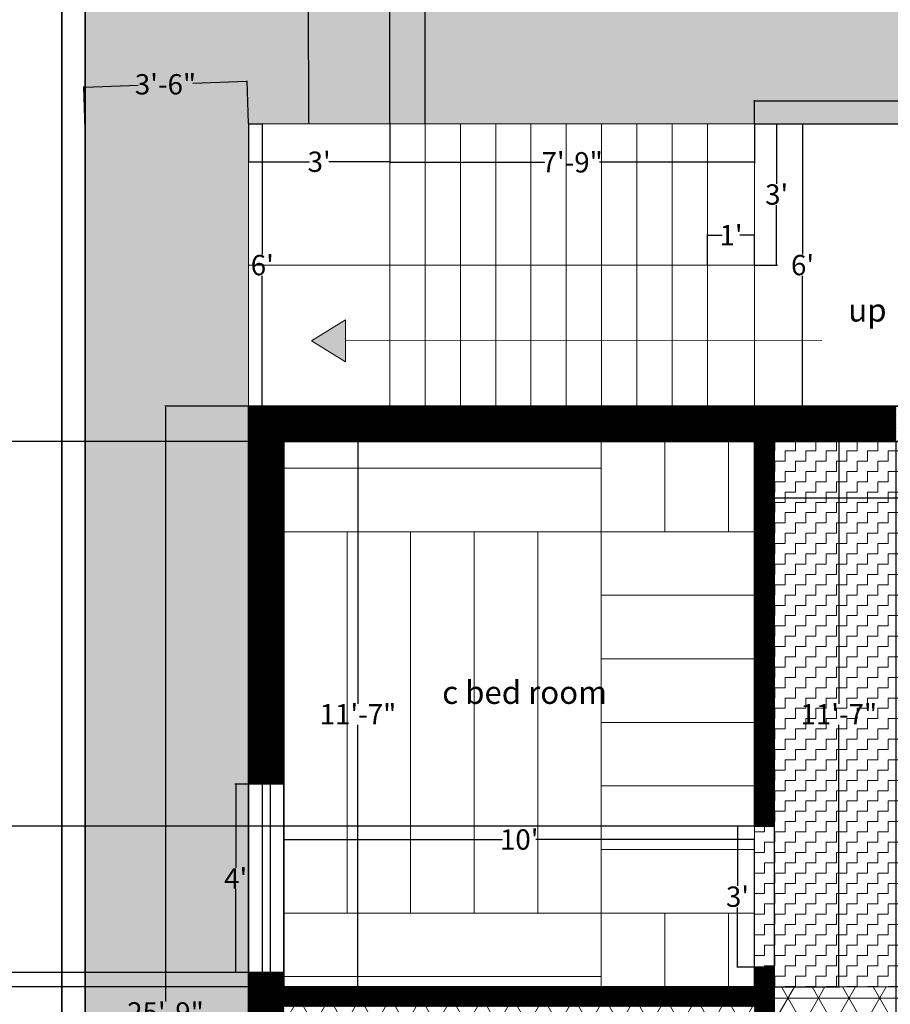
# Model space of a CAD drawing. Units: inches. Extents: x -157 to 1464, y -361 to 1077.
# Tile 5 of 9: x 241 to 463, y 268 to 519. Entities that reach past the tile are written whole.
import ezdxf

# ---------------------------------------------------------------- set-up
doc = ezdxf.new("R2010")
doc.units = ezdxf.units.IN
doc.header["$MEASUREMENT"] = 0
for name, color, linetype, lineweight in [('A-ANNO-DIMS', 2, 'Continuous', 18), ('A-ANNO-SYMB', 7, 'Continuous', 18), ('A-ANNO-SYMB-PATT', 7, 'Continuous', 13), ('A-ANNO-TEXT', 7, 'Continuous', 18), ('A-AREA-IDEN', 7, 'Continuous', 18), ('A-FLOR', 7, 'Continuous', 25), ('A-FLOR-BNDY', 9, 'Continuous', 13), ('A-FLOR-PATT', 8, 'Continuous', 13), ('A-FLOR-STRS', 7, 'Continuous', 18), ('A-WALL', 7, 'Continuous', 35), ('A-WALL-PATT', 252, 'Continuous', 13), ('C-ANNO-DIMS', 2, 'Continuous', 18), ('C-PROP', 7, 'Continuous', 35), ('doors and windows', 33, 'Continuous', 25), ('L-GRND-PATT', 8, 'Continuous', 13)]:
    doc.layers.add(name, color=color, linetype=linetype, lineweight=lineweight)
doc.styles.get("Standard").update_dxf_attribs({"font": 'arial.ttf'})
doc.dimstyles.new('Annotative', dxfattribs={"dimscale": 0, "dimtxt": 5.18, "dimasz": 0.18, "dimexe": 0.18, "dimexo": 0.0625, "dimgap": 0.09, "dimtad": 0, "dimtih": 1, "dimtoh": 1, "dimdec": 0, "dimzin": 0, "dimdsep": 46, "dimlunit": 3, "dimtxsty": 'Standard', "dimcen": 0.09, "dimadec": 0, "dimazin": 0, "dimtfac": 1, "dimtdec": 0, "dimtofl": 0, "dimtmove": 0, "dimatfit": 3, "dimfxl": 1, "dimtolj": 1, "dimtzin": 0, "dimarcsym": 0})

# ---------------------------------------------------------------- blocks, each defined once
blk = doc.blocks.new('*D1')
at = {"layer": 'A-ANNO-DIMS', "color": 0, "lineweight": -2, "transparency": 16777216}
for p, q in [((298.9, 420.86), (277.62, 420.86)), ((277.8, 420.68), (277.8, 269.1)), ((277.8, 112.04), (277.8, 263.63)), ((298.9, 111.86), (277.62, 111.86))]:
    blk.add_line(p, q, dxfattribs=at)
at = {"layer": 'A-ANNO-DIMS', "color": 0, "transparency": 16777216}
for points in [[(277.77, 420.68), (277.83, 420.68), (277.8, 420.86)], [(277.77, 112.04), (277.83, 112.04), (277.8, 111.86)]]:
    blk.add_solid(points, dxfattribs=at)
at = {"layer": 'Defpoints', "color": 0, "transparency": 16777216}
for p in [(298.97, 420.86), (277.8, 111.86), (298.97, 111.86)]:
    blk.add_point(p, dxfattribs=at)
at = {"layer": 'A-ANNO-DIMS', "color": 0, "transparency": 16777216, "insert": (277.8, 266.36), "char_height": 5.18, "attachment_point": 5}
blk.add_mtext('\\A1;25\'-9"', dxfattribs=at)
blk = doc.blocks.new('*D7')
at = {"layer": 'A-ANNO-DIMS', "color": 0, "lineweight": -2, "transparency": 16777216}
for p, q in [((307.97, 272.92), (307.97, 310.62)), ((308.15, 310.44), (363.72, 310.44)), ((427.79, 310.44), (372.21, 310.44)), ((427.97, 272.92), (427.97, 310.62))]:
    blk.add_line(p, q, dxfattribs=at)
at = {"layer": 'A-ANNO-DIMS', "color": 0, "transparency": 16777216}
for points in [[(308.15, 310.47), (308.15, 310.41), (307.97, 310.44)], [(427.79, 310.47), (427.79, 310.41), (427.97, 310.44)]]:
    blk.add_solid(points, dxfattribs=at)
at = {"layer": 'Defpoints', "color": 0, "transparency": 16777216}
for p in [(427.97, 310.44), (307.97, 272.86), (427.97, 272.86)]:
    blk.add_point(p, dxfattribs=at)
at = {"layer": 'A-ANNO-DIMS', "color": 0, "transparency": 16777216, "insert": (367.97, 310.44), "char_height": 5.18, "attachment_point": 5}
blk.add_mtext("\\A1;10'", dxfattribs=at)
blk = doc.blocks.new('*D8')
at = {"layer": 'A-ANNO-DIMS', "color": 0, "lineweight": -2, "transparency": 16777216}
for p, q in [((308.03, 411.86), (327.05, 411.86)), ((326.87, 411.68), (326.87, 345.05)), ((326.87, 273.04), (326.87, 339.67)), ((308.03, 272.86), (327.05, 272.86))]:
    blk.add_line(p, q, dxfattribs=at)
at = {"layer": 'A-ANNO-DIMS', "color": 0, "transparency": 16777216}
for points in [[(326.84, 411.68), (326.9, 411.68), (326.87, 411.86)], [(326.84, 273.04), (326.9, 273.04), (326.87, 272.86)]]:
    blk.add_solid(points, dxfattribs=at)
at = {"layer": 'Defpoints', "color": 0, "transparency": 16777216}
for p in [(307.97, 411.86), (326.87, 411.86), (307.97, 272.86)]:
    blk.add_point(p, dxfattribs=at)
at = {"layer": 'A-ANNO-DIMS', "color": 0, "transparency": 16777216, "insert": (326.87, 342.36), "char_height": 5.18, "attachment_point": 5}
blk.add_mtext('\\A1;11\'-7"', dxfattribs=at)
blk = doc.blocks.new('*D13')
at = {"layer": 'C-ANNO-DIMS', "color": 0, "lineweight": -2, "transparency": 16777216}
for p, q in [((257.27, 643.42), (188.08, 643.42)), ((188.26, 643.24), (188.26, 359.63)), ((188.26, 70.55), (188.26, 354.16)), ((257.27, 70.37), (188.08, 70.37))]:
    blk.add_line(p, q, dxfattribs=at)
at = {"layer": 'C-ANNO-DIMS', "color": 0, "transparency": 16777216}
for points in [[(188.23, 643.24), (188.29, 643.24), (188.26, 643.42)], [(188.23, 70.55), (188.29, 70.55), (188.26, 70.37)]]:
    blk.add_solid(points, dxfattribs=at)
at = {"layer": 'Defpoints', "color": 0, "transparency": 16777216}
for p in [(257.33, 643.42), (188.26, 70.37), (257.33, 70.37)]:
    blk.add_point(p, dxfattribs=at)
at = {"layer": 'C-ANNO-DIMS', "color": 0, "transparency": 16777216, "insert": (188.26, 356.89), "char_height": 5.18, "attachment_point": 5}
blk.add_mtext('\\A1;47\'-9"', dxfattribs=at)
blk = doc.blocks.new('*D18')
at = {"layer": 'A-ANNO-DIMS', "color": 0, "lineweight": -2, "transparency": 16777216}
for p, q in [((298.97, 492.8), (298.97, 483.03)), ((334.97, 492.8), (334.97, 483.03)), ((299.15, 483.21), (314.5, 483.21)), ((334.79, 483.21), (319.44, 483.21))]:
    blk.add_line(p, q, dxfattribs=at)
at = {"layer": 'A-ANNO-DIMS', "color": 0, "transparency": 16777216}
for points in [[(299.15, 483.24), (299.15, 483.18), (298.97, 483.21)], [(334.79, 483.24), (334.79, 483.18), (334.97, 483.21)]]:
    blk.add_solid(points, dxfattribs=at)
at = {"layer": 'Defpoints', "color": 0, "transparency": 16777216}
for p in [(298.97, 492.86), (334.97, 492.86), (334.97, 483.21)]:
    blk.add_point(p, dxfattribs=at)
at = {"layer": 'A-ANNO-DIMS', "color": 0, "transparency": 16777216, "insert": (316.97, 483.21), "char_height": 5.18, "attachment_point": 5}
blk.add_mtext("\\A1;3'", dxfattribs=at)
blk = doc.blocks.new('*D19')
at = {"layer": 'A-ANNO-DIMS', "color": 0, "lineweight": -2, "transparency": 16777216}
for p, q in [((334.97, 492.8), (334.97, 482.88)), ((427.97, 492.8), (427.97, 482.88)), ((335.15, 483.06), (374.51, 483.06)), ((427.79, 483.06), (388.42, 483.06))]:
    blk.add_line(p, q, dxfattribs=at)
at = {"layer": 'A-ANNO-DIMS', "color": 0, "transparency": 16777216}
for points in [[(335.15, 483.09), (335.15, 483.03), (334.97, 483.06)], [(427.79, 483.09), (427.79, 483.03), (427.97, 483.06)]]:
    blk.add_solid(points, dxfattribs=at)
at = {"layer": 'Defpoints', "color": 0, "transparency": 16777216}
for p in [(334.97, 492.86), (427.97, 492.86), (427.97, 483.06)]:
    blk.add_point(p, dxfattribs=at)
at = {"layer": 'A-ANNO-DIMS', "color": 0, "transparency": 16777216, "insert": (381.47, 483.06), "char_height": 5.18, "attachment_point": 5}
blk.add_mtext('\\A1;7\'-9"', dxfattribs=at)
blk = doc.blocks.new('*D20')
at = {"layer": 'A-ANNO-DIMS', "color": 0, "lineweight": -2, "transparency": 16777216}
for p, q in [((299.03, 492.86), (302.65, 492.86)), ((302.47, 492.68), (302.47, 459.6)), ((302.47, 421.04), (302.47, 454.13)), ((299.03, 420.86), (302.65, 420.86))]:
    blk.add_line(p, q, dxfattribs=at)
at = {"layer": 'A-ANNO-DIMS', "color": 0, "transparency": 16777216}
for points in [[(302.44, 492.68), (302.5, 492.68), (302.47, 492.86)], [(302.44, 421.04), (302.5, 421.04), (302.47, 420.86)]]:
    blk.add_solid(points, dxfattribs=at)
at = {"layer": 'Defpoints', "color": 0, "transparency": 16777216}
for p in [(298.97, 492.86), (302.47, 492.86), (298.97, 420.86)]:
    blk.add_point(p, dxfattribs=at)
at = {"layer": 'A-ANNO-DIMS', "color": 0, "transparency": 16777216, "insert": (302.47, 456.86), "char_height": 5.18, "attachment_point": 5}
blk.add_mtext("\\A1;6'", dxfattribs=at)
blk = doc.blocks.new('*D21')
at = {"layer": 'A-ANNO-DIMS', "color": 0, "lineweight": -2, "transparency": 16777216}
for p, q in [((428.03, 492.86), (440.38, 492.86)), ((440.2, 492.68), (440.2, 459.6)), ((440.2, 421.04), (440.2, 454.13)), ((428.03, 420.86), (440.38, 420.86))]:
    blk.add_line(p, q, dxfattribs=at)
at = {"layer": 'A-ANNO-DIMS', "color": 0, "transparency": 16777216}
for points in [[(440.17, 492.68), (440.23, 492.68), (440.2, 492.86)], [(440.17, 421.04), (440.23, 421.04), (440.2, 420.86)]]:
    blk.add_solid(points, dxfattribs=at)
at = {"layer": 'Defpoints', "color": 0, "transparency": 16777216}
for p in [(427.97, 492.86), (427.97, 420.86), (440.2, 420.86)]:
    blk.add_point(p, dxfattribs=at)
at = {"layer": 'A-ANNO-DIMS', "color": 0, "transparency": 16777216, "insert": (440.2, 456.86), "char_height": 5.18, "attachment_point": 5}
blk.add_mtext("\\A1;6'", dxfattribs=at)
blk = doc.blocks.new('*D24')
at = {"layer": 'A-ANNO-DIMS', "color": 0, "lineweight": -2, "transparency": 16777216}
for p, q in [((432.97, 411.8), (432.97, 397.39)), ((587.97, 411.8), (587.97, 397.39)), ((433.15, 397.57), (499.71, 397.57)), ((587.79, 397.57), (521.22, 397.57))]:
    blk.add_line(p, q, dxfattribs=at)
at = {"layer": 'A-ANNO-DIMS', "color": 0, "transparency": 16777216}
for points in [[(433.15, 397.6), (433.15, 397.54), (432.97, 397.57)], [(587.79, 397.6), (587.79, 397.54), (587.97, 397.57)]]:
    blk.add_solid(points, dxfattribs=at)
at = {"layer": 'Defpoints', "color": 0, "transparency": 16777216}
for p in [(432.97, 411.86), (587.97, 411.86), (587.97, 397.57)]:
    blk.add_point(p, dxfattribs=at)
at = {"layer": 'A-ANNO-DIMS', "color": 0, "transparency": 16777216, "insert": (510.47, 397.57), "char_height": 5.18, "attachment_point": 5}
blk.add_mtext('\\A1;12\'-11"', dxfattribs=at)
blk = doc.blocks.new('*D25')
at = {"layer": 'A-ANNO-DIMS', "color": 0, "lineweight": -2, "transparency": 16777216}
for p, q in [((433.03, 411.86), (449.62, 411.86)), ((449.44, 411.68), (449.44, 345.05)), ((449.44, 273.04), (449.44, 339.67)), ((433.03, 272.86), (449.62, 272.86))]:
    blk.add_line(p, q, dxfattribs=at)
at = {"layer": 'A-ANNO-DIMS', "color": 0, "transparency": 16777216}
for points in [[(449.41, 411.68), (449.47, 411.68), (449.44, 411.86)], [(449.41, 273.04), (449.47, 273.04), (449.44, 272.86)]]:
    blk.add_solid(points, dxfattribs=at)
at = {"layer": 'Defpoints', "color": 0, "transparency": 16777216}
for p in [(432.97, 411.86), (432.97, 272.86), (449.44, 272.86)]:
    blk.add_point(p, dxfattribs=at)
at = {"layer": 'A-ANNO-DIMS', "color": 0, "transparency": 16777216, "insert": (449.44, 342.36), "char_height": 5.18, "attachment_point": 5}
blk.add_mtext('\\A1;11\'-7"', dxfattribs=at)
blk = doc.blocks.new('*D34')
at = {"layer": 'A-ANNO-DIMS', "color": 0, "lineweight": -2, "transparency": 16777216}
for p, q in [((302.4, 324.53), (295.51, 324.53)), ((295.69, 324.35), (295.69, 303.21)), ((295.69, 276.71), (295.69, 297.85)), ((302.4, 276.53), (295.51, 276.53))]:
    blk.add_line(p, q, dxfattribs=at)
at = {"layer": 'A-ANNO-DIMS', "color": 0, "transparency": 16777216}
for points in [[(295.66, 324.35), (295.72, 324.35), (295.69, 324.53)], [(295.66, 276.71), (295.72, 276.71), (295.69, 276.53)]]:
    blk.add_solid(points, dxfattribs=at)
at = {"layer": 'Defpoints', "color": 0, "transparency": 16777216}
for p in [(302.47, 324.53), (295.69, 276.53), (302.47, 276.53)]:
    blk.add_point(p, dxfattribs=at)
at = {"layer": 'A-ANNO-DIMS', "color": 0, "transparency": 16777216, "insert": (295.69, 300.53), "char_height": 5.18, "attachment_point": 5}
blk.add_mtext("\\A1;4'", dxfattribs=at)
blk = doc.blocks.new('*D36')
at = {"layer": 'A-ANNO-DIMS', "color": 0, "lineweight": -2, "transparency": 16777216}
for p, q in [((415.97, 456.92), (415.97, 464.68)), ((416.15, 464.5), (419.74, 464.5)), ((427.79, 464.5), (424.2, 464.5)), ((427.97, 456.92), (427.97, 464.68))]:
    blk.add_line(p, q, dxfattribs=at)
at = {"layer": 'A-ANNO-DIMS', "color": 0, "transparency": 16777216}
for points in [[(416.15, 464.53), (416.15, 464.47), (415.97, 464.5)], [(427.79, 464.53), (427.79, 464.47), (427.97, 464.5)]]:
    blk.add_solid(points, dxfattribs=at)
at = {"layer": 'Defpoints', "color": 0, "transparency": 16777216}
for p in [(427.97, 464.5), (415.97, 456.86), (427.97, 456.86)]:
    blk.add_point(p, dxfattribs=at)
at = {"layer": 'A-ANNO-DIMS', "color": 0, "transparency": 16777216, "insert": (421.97, 464.5), "char_height": 5.18, "attachment_point": 5}
blk.add_mtext("\\A1;1'", dxfattribs=at)
blk = doc.blocks.new('*D37')
at = {"layer": 'A-ANNO-DIMS', "color": 0, "lineweight": -2, "transparency": 16777216}
for p, q in [((428.03, 492.86), (433.78, 492.86)), ((433.6, 492.68), (433.6, 477.6)), ((433.6, 457.04), (433.6, 472.12)), ((428.03, 456.86), (433.78, 456.86))]:
    blk.add_line(p, q, dxfattribs=at)
at = {"layer": 'A-ANNO-DIMS', "color": 0, "transparency": 16777216}
for points in [[(433.57, 492.68), (433.63, 492.68), (433.6, 492.86)], [(433.57, 457.04), (433.63, 457.04), (433.6, 456.86)]]:
    blk.add_solid(points, dxfattribs=at)
at = {"layer": 'Defpoints', "color": 0, "transparency": 16777216}
for p in [(427.97, 492.86), (427.97, 456.86), (433.6, 456.86)]:
    blk.add_point(p, dxfattribs=at)
at = {"layer": 'A-ANNO-DIMS', "color": 0, "transparency": 16777216, "insert": (433.6, 474.86), "char_height": 5.18, "attachment_point": 5}
blk.add_mtext("\\A1;3'", dxfattribs=at)
blk = doc.blocks.new('*D50')
at = {"layer": 'A-ANNO-DIMS', "color": 0, "lineweight": -2, "transparency": 16777216}
for p, q in [((427.9, 313.86), (423.44, 313.86)), ((423.62, 313.68), (423.62, 298.6)), ((423.62, 278.04), (423.62, 293.12)), ((427.9, 277.86), (423.44, 277.86))]:
    blk.add_line(p, q, dxfattribs=at)
at = {"layer": 'A-ANNO-DIMS', "color": 0, "transparency": 16777216}
for points in [[(423.59, 313.68), (423.65, 313.68), (423.62, 313.86)], [(423.59, 278.04), (423.65, 278.04), (423.62, 277.86)]]:
    blk.add_solid(points, dxfattribs=at)
at = {"layer": 'Defpoints', "color": 0, "transparency": 16777216}
for p in [(427.97, 313.86), (423.62, 277.86), (427.97, 277.86)]:
    blk.add_point(p, dxfattribs=at)
at = {"layer": 'A-ANNO-DIMS', "color": 0, "transparency": 16777216, "insert": (423.62, 295.86), "char_height": 5.18, "attachment_point": 5}
blk.add_mtext("\\A1;3'", dxfattribs=at)
blk = doc.blocks.new('*D52')
at = {"layer": 'C-ANNO-DIMS', "color": 0, "lineweight": -2, "transparency": 16777216}
for p, q in [((298.45, 643.58), (313.95, 643.64)), ((313.77, 643.46), (314.04, 570.97)), ((314.34, 493.1), (314.06, 565.59)), ((299.03, 492.86), (314.52, 492.92))]:
    blk.add_line(p, q, dxfattribs=at)
at = {"layer": 'C-ANNO-DIMS', "color": 0, "transparency": 16777216}
for points in [[(313.8, 643.46), (313.74, 643.46), (313.77, 643.64)], [(314.37, 493.1), (314.31, 493.1), (314.34, 492.92)]]:
    blk.add_solid(points, dxfattribs=at)
at = {"layer": 'Defpoints', "color": 0, "transparency": 16777216}
for p in [(298.39, 643.58), (313.77, 643.64), (298.97, 492.86)]:
    blk.add_point(p, dxfattribs=at)
at = {"layer": 'C-ANNO-DIMS', "color": 0, "transparency": 16777216, "insert": (314.05, 568.28), "char_height": 5.18, "attachment_point": 5}
blk.add_mtext('\\A1;12\'-7"', dxfattribs=at)
blk = doc.blocks.new('*D53')
at = {"layer": 'C-ANNO-DIMS', "color": 0, "lineweight": -2, "transparency": 16777216}
for p, q in [((257.33, 491.52), (256.96, 502.43)), ((257.15, 502.26), (270.81, 502.71)), ((298.42, 503.64), (284.76, 503.18)), ((298.96, 492.92), (298.6, 503.83))]:
    blk.add_line(p, q, dxfattribs=at)
at = {"layer": 'C-ANNO-DIMS', "color": 0, "transparency": 16777216}
for points in [[(257.15, 502.29), (257.15, 502.23), (256.97, 502.25)], [(298.42, 503.67), (298.43, 503.61), (298.6, 503.65)]]:
    blk.add_solid(points, dxfattribs=at)
at = {"layer": 'Defpoints', "color": 0, "transparency": 16777216}
for p in [(256.97, 502.25), (298.97, 492.86), (257.33, 491.46)]:
    blk.add_point(p, dxfattribs=at)
at = {"layer": 'C-ANNO-DIMS', "color": 0, "transparency": 16777216, "insert": (277.79, 502.95), "char_height": 5.18, "attachment_point": 5}
blk.add_mtext('\\A1;3\'-6"', dxfattribs=at)
blk = doc.blocks.new('*D57')
at = {"layer": 'A-ANNO-DIMS', "color": 0, "lineweight": -2, "transparency": 16777216}
for p, q in [((427.97, 492.92), (427.97, 498.91)), ((428.15, 498.73), (539.44, 498.73)), ((668.79, 498.73), (557.5, 498.73)), ((668.97, 492.92), (668.97, 498.91))]:
    blk.add_line(p, q, dxfattribs=at)
at = {"layer": 'A-ANNO-DIMS', "color": 0, "transparency": 16777216}
for points in [[(428.15, 498.76), (428.15, 498.7), (427.97, 498.73)], [(668.79, 498.76), (668.79, 498.7), (668.97, 498.73)]]:
    blk.add_solid(points, dxfattribs=at)
at = {"layer": 'Defpoints', "color": 0, "transparency": 16777216}
for p in [(668.97, 498.73), (427.97, 492.86), (668.97, 492.86)]:
    blk.add_point(p, dxfattribs=at)
at = {"layer": 'A-ANNO-DIMS', "color": 0, "transparency": 16777216, "insert": (548.47, 498.73), "char_height": 5.18, "attachment_point": 5}
blk.add_mtext('\\A1;20\'-1"', dxfattribs=at)
blk = doc.blocks.new('WIN-48x9')
for p, q in [((9, 48), (0, 48)), ((0, 48), (0, 0)), ((3.5, 48), (3.5, 0)), ((5.5, 48), (5.5, 0)), ((9, 48), (9, 0)), ((9, 0), (0, 0))]:
    blk.add_line(p, q)
blk = doc.blocks.new('*D72')
at = {"layer": 'A-ANNO-DIMS', "color": 0, "lineweight": -2, "transparency": 16777216}
for p, q in [((298.9, 276.53), (-141.39, 276.53)), ((-141.21, 276.53), (-141.21, 276.71)), ((-141.21, 276.71), (-141.03, 276.71)), ((-141.21, 273.04), (-141.21, 276.35)), ((307.9, 272.86), (-141.39, 272.86))]:
    blk.add_line(p, q, dxfattribs=at)
at = {"layer": 'A-ANNO-DIMS', "color": 0, "transparency": 16777216}
for points in [[(-141.24, 276.35), (-141.18, 276.35), (-141.21, 276.53)], [(-141.24, 273.04), (-141.18, 273.04), (-141.21, 272.86)]]:
    blk.add_solid(points, dxfattribs=at)
at = {"layer": 'Defpoints', "color": 0, "transparency": 16777216}
for p in [(-141.21, 276.53), (298.97, 276.53), (307.97, 272.86)]:
    blk.add_point(p, dxfattribs=at)
at = {"layer": 'A-ANNO-DIMS', "color": 0, "transparency": 16777216, "insert": (-128.02, 276.71), "char_height": 5.18, "attachment_point": 5}
blk.add_mtext('\\A1;0\'-3 1/2"', dxfattribs=at)
blk = doc.blocks.new('*D73')
at = {"layer": 'A-ANNO-DIMS', "color": 0, "lineweight": -2, "transparency": 16777216}
for p, q in [((432.97, 411.8), (432.97, -357.73)), ((463.95, 411.8), (463.95, -357.73)), ((433.15, -357.55), (441.44, -357.55)), ((463.77, -357.55), (455.48, -357.55))]:
    blk.add_line(p, q, dxfattribs=at)
at = {"layer": 'A-ANNO-DIMS', "color": 0, "transparency": 16777216}
for points in [[(433.15, -357.52), (433.15, -357.58), (432.97, -357.55)], [(463.77, -357.52), (463.77, -357.58), (463.95, -357.55)]]:
    blk.add_solid(points, dxfattribs=at)
at = {"layer": 'Defpoints', "color": 0, "transparency": 16777216}
for p in [(432.97, 411.86), (463.95, 411.86), (463.95, -357.55)]:
    blk.add_point(p, dxfattribs=at)
at = {"layer": 'A-ANNO-DIMS', "color": 0, "transparency": 16777216, "insert": (448.46, -357.55), "char_height": 5.18, "attachment_point": 5}
blk.add_mtext('\\A1;2\'-7"', dxfattribs=at)
blk = doc.blocks.new('*D77')
at = {"layer": 'A-ANNO-DIMS', "color": 0, "lineweight": -2, "transparency": 16777216}
for p, q in [((427.9, 411.86), (-141.39, 411.86)), ((-141.21, 411.68), (-141.21, 365.6)), ((-141.21, 314.04), (-141.21, 360.13)), ((427.9, 313.86), (-141.39, 313.86))]:
    blk.add_line(p, q, dxfattribs=at)
at = {"layer": 'A-ANNO-DIMS', "color": 0, "transparency": 16777216}
for points in [[(-141.24, 411.68), (-141.18, 411.68), (-141.21, 411.86)], [(-141.24, 314.04), (-141.18, 314.04), (-141.21, 313.86)]]:
    blk.add_solid(points, dxfattribs=at)
at = {"layer": 'Defpoints', "color": 0, "transparency": 16777216}
for p in [(-141.21, 411.86), (427.97, 411.86), (427.97, 313.86)]:
    blk.add_point(p, dxfattribs=at)
at = {"layer": 'A-ANNO-DIMS', "color": 0, "transparency": 16777216, "insert": (-141.21, 362.86), "char_height": 5.18, "attachment_point": 5}
blk.add_mtext('\\A1;8\'-2"', dxfattribs=at)
blk = doc.blocks.new('*D80')
at = {"layer": 'A-ANNO-DIMS', "color": 0, "lineweight": -2, "transparency": 16777216}
for p, q in [((334.97, 492.92), (334.97, 1069.66)), ((335.15, 1069.48), (343.79, 1069.48)), ((343.97, 492.92), (343.97, 1069.66)), ((343.97, 1069.48), (344.15, 1069.48))]:
    blk.add_line(p, q, dxfattribs=at)
at = {"layer": 'A-ANNO-DIMS', "color": 0, "transparency": 16777216}
for points in [[(335.15, 1069.51), (335.15, 1069.45), (334.97, 1069.48)], [(343.79, 1069.51), (343.79, 1069.45), (343.97, 1069.48)]]:
    blk.add_solid(points, dxfattribs=at)
at = {"layer": 'Defpoints', "color": 0, "transparency": 16777216}
for p in [(343.97, 1069.48), (334.97, 492.86), (343.97, 492.86)]:
    blk.add_point(p, dxfattribs=at)
at = {"layer": 'A-ANNO-DIMS', "color": 0, "transparency": 16777216, "insert": (351.12, 1069.48), "char_height": 5.18, "attachment_point": 5}
blk.add_mtext('\\A1;0\'-9"', dxfattribs=at)

msp = doc.modelspace()

# ---------------------------------------------------------------- hatches: boundary and pattern name
at = {"layer": 'A-ANNO-SYMB-PATT'}
h = msp.add_hatch(color=256, dxfattribs=at)
h.dxf.hatch_style = 1
h.paths.add_polyline_path([(323.7, 442.93), (315.01, 437.58), (323.7, 432.23)])
at = {"layer": 'A-FLOR-PATT'}
h = msp.add_hatch(dxfattribs=at)
h.set_pattern_fill('AR-PARQ1', color=256, scale=8.1)
h.paths.add_polyline_path([(427.97, 411.86), (307.97, 411.86), (307.97, 272.86), (427.97, 272.86), (427.97, 277.86), (427.97, 313.86)])
h = msp.add_hatch(dxfattribs=at)
h.set_pattern_fill('ZIGZAG', color=256, scale=21)
h.set_pattern_definition([(0, (0, 0), (2.625, 2.625), [2.625, -2.625]), (90, (2.625, 0), (-2.625, 2.625), [2.625, -2.625])])
h.paths.add_polyline_path([(587.97, 272.86), (587.97, 369.86), (587.97, 405.86), (587.97, 411.86), (582.97, 411.86), (546.97, 411.86), (432.97, 411.86), (432.97, 313.86), (427.97, 313.86), (427.97, 277.86), (432.97, 277.86), (432.97, 272.86), (480.97, 272.86)])
h.paths.add_polyline_path([(497.45, 333.85), (513.07, 333.85), (513.07, 345.88), (497.45, 345.88)], flags=24)
h = msp.add_hatch(dxfattribs=at)
h.set_pattern_fill('NET3', color=256, scale=54)
h.paths.add_polyline_path([(563.97, 267.86), (480.97, 267.86), (480.97, 272.86), (432.97, 272.86), (432.97, 262.86), (427.97, 262.86), (427.97, 267.86), (307.97, 267.86), (307.97, 120.86), (427.97, 120.86), (427.97, 226.86), (432.97, 226.86), (432.97, 203.86), (438.97, 203.86), (468.97, 203.86), (485.97, 203.86), (485.97, 144.86), (563.97, 144.86)])
h.paths.add_polyline_path([(507.66, 186.06), (540.97, 186.06), (540.97, 198.1), (507.66, 198.1)], flags=24)
h.paths.add_polyline_path([(343.4, 209.88), (389.84, 209.88), (389.84, 221.92), (343.4, 221.92)], flags=24)
at = {"layer": 'A-WALL-PATT'}
h = msp.add_hatch(dxfattribs=at)
h.set_pattern_fill('ANSI31', color=256)
h.set_pattern_definition([(45, (213.19381, 103.60139), (-0.088388348, 0.088388348), [])])
h.paths.add_polyline_path([(307.97, 267.86), (427.97, 267.86), (427.97, 262.86), (432.97, 262.86), (432.97, 277.86), (427.97, 277.86), (427.97, 272.86), (307.97, 272.86), (307.97, 276.53), (298.97, 276.53), (298.97, 194.36), (307.97, 194.36)])
h.paths.add_polyline_path([(307.97, 411.86), (427.97, 411.86), (427.97, 313.86), (432.97, 313.86), (432.97, 411.86), (463.95, 411.86), (463.95, 420.86), (298.97, 420.86), (298.97, 324.53), (307.97, 324.53)])
h.paths.add_polyline_path([(511.95, 420.86), (511.95, 411.86), (546.97, 411.86), (546.97, 420.86)])
h.paths.add_polyline_path([(587.97, 411.86), (587.97, 405.86), (596.97, 405.86), (596.97, 420.86), (582.97, 420.86), (582.97, 411.86)])
h.paths.add_polyline_path([(587.97, 369.86), (587.97, 324), (596.97, 324), (596.97, 369.86)])
h.paths.add_polyline_path([(596.97, 276), (587.97, 276), (587.97, 272.86), (480.97, 272.86), (480.97, 267.86), (587.97, 267.86), (587.97, 206.9), (596.97, 206.9)])
h.paths.add_polyline_path([(587.97, 120.86), (485.97, 120.86), (485.97, 203.86), (468.97, 203.86), (468.97, 198.86), (480.97, 198.86), (480.97, 120.86), (465.97, 120.86), (465.97, 111.86), (596.97, 111.86), (596.97, 158.9), (587.97, 158.9)])
h.paths.add_polyline_path([(427.97, 120.86), (307.97, 120.86), (307.97, 146.36), (298.97, 146.36), (298.97, 111.86), (447.97, 111.86), (447.97, 120.86), (432.97, 120.86), (432.97, 198.86), (438.97, 198.86), (438.97, 203.86), (432.97, 203.86), (432.97, 226.86), (427.97, 226.86)])
at = {"layer": 'L-GRND-PATT'}
h = msp.add_hatch(dxfattribs=at)
h.set_pattern_fill('GRAVEL', color=256, scale=26)
h.set_pattern_definition([(228.01279, (18.72, 26), (-208, -234), [3.49794, -346.2963]), (184.96974, (16.38, 23.4), (312, 26), [6.00257, -594.25404]), (132.51045, (10.4, 22.88), (260, -286), [4.2325, -419.01685]), (267.27369, (0.26, 16.38), (26, 520), [5.4662, -541.1525]), (292.83365, (0, 10.92), (-130, 312), [5.36003, -530.6437]), (357.27369, (2.08, 5.98), (-520, 26), [5.4662, -541.1525]), (37.69424, (7.54, 5.72), (-338, -260), [7.22875, -715.64606]), (72.25533, (13.26, 10.14), (182, 572), [6.8247, -675.64436]), (121.42957, (15.34, 16.64), (-208, 338), [5.4847, -542.9859]), (175.23636, (12.48, 21.32), (286, -26), [6.26163, -306.81983]), (222.39744, (6.24, 21.84), (-312, -286), [8.09765, -801.66775]), (138.81407, (26, 16.12), (-182, 156), [2.76383, -273.61997]), (171.46923, (23.92, 17.94), (338, -52), [5.25816, -520.5593]), (225, (18.72, 18.72), (-3e-15, -26), [3.67695, -33.0926]), (203.1986, (16.9, 21.84), (130, 52), [1.9801, -196.03]), (291.8014, (15.08, 21.06), (-26, 78), [2.8003, -137.214]), (30.96376, (16.12, 18.46), (78, 52), [4.54815, -147.0566]), (161.56505, (20.02, 20.8), (52, -26), [3.28877, -78.93045]), (16.38954, (0, 21.06), (260, 78), [4.6072, -456.11397]), (70.34618, (4.42, 22.36), (-104, -286), [3.8652, -382.6526]), (293.1986, (20.02, 26), (-52, 130), [3.9602, -194.0499]), (343.61046, (21.58, 22.36), (-260, 78), [4.6072, -456.11397]), (339.44395, (0, 4.94), (-130, 52), [4.4429, -217.7012]), (294.77514, (4.16, 3.38), (-130, 286), [3.72263, -368.5407]), (66.8014, (20.28, 0), (52, 130), [3.9602, -194.0499]), (17.35402, (21.84, 3.64), (-338, -104), [4.3584, -431.481]), (69.44395, (7.54, 0), (-52, -130), [2.22144, -219.92266]), (101.30993, (18.72, 0), (-26, 104), [1.32574, -131.24877]), (165.96376, (18.46, 1.3), (78, -26), [5.36003, -101.8407]), (186.009, (13.26, 2.6), (260, 26), [4.9673, -491.762]), (303.6901, (16.12, 16.12), (-26, 52), [3.7498, -89.99456]), (353.15723, (18.2, 13), (442, -52), [6.54664, -648.11663]), (60.9454, (24.7, 12.22), (-104, -182), [2.67686, -265.00953]), (90, (26, 14.56), (-26, 26), [1.56, -24.44]), (120.25644, (12.74, 3.38), (104, -182), [3.61202, -357.5915]), (48.01279, (10.92, 6.5), (208, 234), [6.99587, -342.79835]), (0, (15.6, 11.7), (26, 26), [6.76, -19.24]), (325.30485, (22.36, 11.7), (260, -182), [4.11096, -406.98513]), (254.0546, (25.74, 9.36), (-26, -104), [3.78565, -185.4972]), (207.64598, (24.7, 5.72), (-494, -260), [6.1637, -610.20633]), (175.42608, (19.24, 2.86), (-338, 26), [6.52077, -645.5559])])
h.paths.add_polyline_path([(856.57, 645.71), (257.33, 643.42), (257.33, 70.37), (856.57, 72.66)])
h.paths.add_polyline_path([(668.97, 111.86), (596.97, 111.86), (298.97, 111.86), (298.97, 420.86), (298.97, 492.86), (427.97, 492.86), (668.97, 492.86)], flags=16)
h.paths.add_polyline_path([(842.44, 305.24), (842.44, 199.78), (692.18, 199.78), (692.18, 305.24)], flags=16)
h.paths.add_polyline_path([(596.97, 369.86), (596.97, 158.9), (587.97, 158.9), (587.97, 120.86), (485.97, 120.86), (485.97, 203.86), (468.97, 203.86), (468.97, 198.86), (480.97, 198.86), (480.97, 120.86), (465.97, 120.86), (465.97, 111.86), (447.97, 111.86), (447.97, 120.86), (432.97, 120.86), (432.97, 198.86), (438.97, 198.86), (438.97, 203.86), (432.97, 203.86), (432.97, 226.86), (427.97, 226.86), (427.97, 120.86), (307.97, 120.86), (307.97, 146.36), (298.97, 146.36), (298.97, 194.36), (307.97, 194.36), (307.97, 267.86), (427.97, 267.86), (427.97, 262.86), (432.97, 262.86), (432.97, 277.86), (427.97, 277.86), (427.97, 272.86), (307.97, 272.86), (307.97, 276.53), (298.97, 276.53), (298.97, 324.53), (307.97, 324.53), (307.97, 411.86), (427.97, 411.86), (427.97, 313.86), (432.97, 313.86), (432.97, 411.86), (463.95, 411.86), (463.95, 420.86), (334.97, 420.86), (334.97, 456.86), (427.97, 456.86), (427.97, 420.86), (546.97, 420.86), (582.97, 420.86), (596.97, 420.86), (596.97, 405.86)], flags=0)
h.paths.add_polyline_path([(596.97, 369.86), (587.97, 369.86), (587.97, 324), (596.97, 324), (596.97, 276), (587.97, 276), (587.97, 369.86), (587.97, 405.86), (587.97, 411.86), (582.97, 411.86), (546.97, 411.86), (546.97, 420.86), (564.97, 416.36), (582.97, 420.86), (582.97, 411.86), (587.97, 411.86), (587.97, 405.86), (596.97, 405.86), (592.47, 387.86)], flags=0)
h.paths.add_polyline_path([(468.97, 203.86), (468.97, 198.86), (438.97, 198.86), (438.97, 203.86)], flags=0)
h.paths.add_polyline_path([(267.35, 260.99), (288.37, 260.99), (288.37, 271.66), (267.35, 271.66)], flags=24)
h.paths.add_polyline_path([(435.51, 88.48), (460.55, 88.48), (460.55, 99.15), (435.51, 99.15)], flags=24)
h.paths.add_polyline_path([(315.69, 188.99), (336.72, 188.99), (336.72, 199.66), (315.69, 199.66)], flags=8)
h.paths.add_polyline_path([(361.73, 141.9), (373.75, 141.9), (373.75, 152.57), (361.73, 152.57)], flags=8)
h.paths.add_polyline_path([(430.38, 154.49), (447.38, 154.49), (447.38, 165.16), (430.38, 165.16)], flags=8)
h.paths.add_polyline_path([(451.09, 165.32), (468.09, 165.32), (468.09, 175.99), (451.09, 175.99)], flags=8)
h.paths.add_polyline_path([(361.73, 305.06), (373.75, 305.06), (373.75, 315.74), (361.73, 315.74)], flags=8)
h.paths.add_polyline_path([(316.13, 336.94), (337.15, 336.94), (337.15, 347.62), (316.13, 347.62)], flags=8)
h.paths.add_polyline_path([(484.07, 423.56), (492.07, 423.56), (492.07, 434.24), (484.07, 434.24)], flags=8)
h.paths.add_polyline_path([(560.99, 428.52), (568.98, 428.52), (568.98, 439.19), (560.99, 439.19)], flags=8)
h.paths.add_polyline_path([(528.49, 131.95), (545.49, 131.95), (545.49, 142.62), (528.49, 142.62)], flags=8)
h.paths.add_polyline_path([(564.53, 188.99), (585.55, 188.99), (585.55, 199.66), (564.53, 199.66)], flags=8)

# ---------------------------------------------------------------- linework, layer by layer
at = {"layer": 'A-ANNO-SYMB'}
for p, q in [((315.01, 437.58), (323.7, 442.93)), ((323.7, 442.93), (323.7, 432.23)), ((315.01, 437.58), (323.7, 432.23)), ((445.08, 437.68), (323.7, 437.58))]:
    msp.add_line(p, q, dxfattribs=at)
at = {"layer": 'A-FLOR'}
msp.add_line((427.97, 492.86), (668.97, 492.86), dxfattribs=at)
at = {"layer": 'A-FLOR-BNDY'}
for p, q in [((427.97, 313.86), (427.97, 277.86)), ((480.97, 272.86), (432.97, 272.86))]:
    msp.add_line(p, q, dxfattribs=at)
at = {"layer": 'A-FLOR-STRS'}
for p, q in [((298.97, 420.86), (298.97, 492.86)), ((427.97, 492.86), (298.97, 492.86)), ((334.97, 420.86), (334.97, 492.86)), ((343.97, 420.86), (343.97, 492.86)), ((352.97, 420.86), (352.97, 492.86)), ((361.97, 420.86), (361.97, 492.86)), ((370.97, 420.86), (370.97, 492.86)), ((379.97, 420.86), (379.97, 492.86)), ((388.97, 420.86), (388.97, 492.86)), ((388.97, 420.86), (388.97, 492.86)), ((397.97, 420.86), (397.97, 492.86)), ((406.97, 420.86), (406.97, 492.86)), ((415.97, 420.86), (415.97, 492.86)), ((427.97, 492.86), (427.97, 420.86)), ((298.97, 456.86), (427.97, 456.86))]:
    msp.add_line(p, q, dxfattribs=at)
at = {"layer": 'A-WALL'}
for p, q in [((298.97, 111.86), (298.97, 420.86)), ((298.97, 420.86), (546.97, 420.86)), ((307.97, 411.86), (427.97, 411.86)), ((307.97, 272.86), (307.97, 411.86)), ((427.97, 313.86), (427.97, 411.86)), ((432.97, 411.86), (546.97, 411.86)), ((432.97, 313.86), (432.97, 411.86)), ((427.97, 313.86), (432.97, 313.86)), ((427.97, 272.86), (427.97, 277.86)), ((427.97, 277.86), (432.97, 277.86)), ((432.97, 262.86), (432.97, 277.86)), ((307.97, 272.86), (427.97, 272.86))]:
    msp.add_line(p, q, dxfattribs=at)
at = {"layer": 'C-PROP'}
msp.add_lwpolyline([(862.57, 615.42), (862.57, 651.74), (251.33, 649.4), (251.33, 64.34), (862.57, 66.68), (862.57, 519.42)], dxfattribs=at)
msp.add_lwpolyline([(257.33, 70.37), (856.57, 72.66), (856.57, 645.71), (257.33, 643.42)], close=True, dxfattribs=at)

# ---------------------------------------------------------------- block references
at = {"layer": 'doors and windows'}
msp.add_blockref('WIN-48x9', (298.97, 276.53), dxfattribs=at)

# ---------------------------------------------------------------- texts
at = {"layer": 'A-ANNO-TEXT', "insert": (451.85, 448.31), "char_height": 5.84, "attachment_point": 1}
msp.add_mtext_dynamic_manual_height_columns('up', width=87.358, gutter_width=29.2, heights=[13.12], dxfattribs=at)
at = {"layer": 'A-AREA-IDEN', "insert": (348.34, 350.85), "char_height": 5.84, "attachment_point": 1}
msp.add_mtext_dynamic_manual_height_columns('c bed room', width=87.358, gutter_width=29.2, heights=[13.12], dxfattribs=at)

# ---------------------------------------------------------------- dimensions: what is measured, and where the dimension line sits
at = {"layer": 'A-ANNO-DIMS'}
for base, p1, p2, override, picture, middle in [((343.97, 1069.48), (334.97, 492.86), (343.97, 492.86), {"dimscale": 1, "dimdec": 1, "dimzin": 1, "dimlunit": 4, "dimfrac": 2}, '*D80', (351.12, 1069.48)), ((668.97, 498.73), (427.97, 492.86), (668.97, 492.86), {"dimclrd": 0, "dimclre": 0, "dimclrt": 0}, '*D57', (548.47, 498.73)), ((334.97, 483.21), (298.97, 492.86), (334.97, 492.86), {"dimclrd": 0, "dimclre": 0, "dimclrt": 0}, '*D18', (316.97, 483.21)), ((427.97, 483.06), (334.97, 492.86), (427.97, 492.86), {"dimclrd": 0, "dimclre": 0, "dimclrt": 0}, '*D19', (381.47, 483.06)), ((427.97, 464.5), (415.97, 456.86), (427.97, 456.86), {"dimclrd": 0, "dimclre": 0, "dimclrt": 0}, '*D36', (421.97, 464.5)), ((587.97, 397.57), (432.97, 411.86), (587.97, 411.86), {"dimclrd": 0, "dimclre": 0, "dimclrt": 0}, '*D24', (510.47, 397.57)), ((463.95, -357.55), (432.97, 411.86), (463.95, 411.86), {"dimscale": 1, "dimdec": 1, "dimzin": 1, "dimlunit": 4, "dimfrac": 2}, '*D73', (448.46, -357.55)), ((427.97, 310.44), (307.97, 272.86), (427.97, 272.86), {"dimclrd": 0, "dimclre": 0, "dimclrt": 0}, '*D7', (367.97, 310.44))]:
    dim = msp.add_linear_dim(base=base, p1=p1, p2=p2, dimstyle='Annotative', override=override, dxfattribs=at)
    dim.commit()
    dim.dimension.update_dxf_attribs({"geometry": picture, "text_midpoint": middle})
for base, p1, p2, override, picture, middle in [((302.47, 492.86), (298.97, 420.86), (298.97, 492.86), {"dimclrd": 0, "dimclre": 0, "dimclrt": 0}, '*D20', (302.47, 456.86)), ((440.2, 420.86), (427.97, 492.86), (427.97, 420.86), {"dimclrd": 0, "dimclre": 0, "dimclrt": 0}, '*D21', (440.2, 456.86)), ((433.6, 456.86), (427.97, 492.86), (427.97, 456.86), {"dimclrd": 0, "dimclre": 0, "dimclrt": 0}, '*D37', (433.6, 474.86)), ((277.8, 111.86), (298.97, 420.86), (298.97, 111.86), {"dimclrd": 0, "dimclre": 0, "dimclrt": 0}, '*D1', (277.8, 266.36)), ((-141.21, 411.86), (427.97, 313.86), (427.97, 411.86), {"dimscale": 1, "dimdec": 1, "dimzin": 1, "dimlunit": 4, "dimfrac": 2}, '*D77', (-141.21, 362.86)), ((326.87, 411.86), (307.97, 272.86), (307.97, 411.86), {"dimclrd": 0, "dimclre": 0, "dimclrt": 0}, '*D8', (326.87, 342.36)), ((449.44, 272.86), (432.97, 411.86), (432.97, 272.86), {"dimclrd": 0, "dimclre": 0, "dimclrt": 0}, '*D25', (449.44, 342.36)), ((295.69, 276.53), (302.47, 324.53), (302.47, 276.53), {"dimclrd": 0, "dimclre": 0, "dimclrt": 0}, '*D34', (295.69, 300.53)), ((423.62, 277.86), (427.97, 313.86), (427.97, 277.86), {"dimclrd": 0, "dimclre": 0, "dimclrt": 0}, '*D50', (423.62, 295.86)), ((-141.21, 276.53), (307.97, 272.86), (298.97, 276.53), {"dimscale": 1, "dimdec": 1, "dimzin": 1, "dimlunit": 4, "dimfrac": 2}, '*D72', (-128.02, 276.71))]:
    dim = msp.add_linear_dim(base=base, p1=p1, p2=p2, angle=90, dimstyle='Annotative', override=override, dxfattribs=at)
    dim.commit()
    dim.dimension.update_dxf_attribs({"geometry": picture, "text_midpoint": middle})
at = {"layer": 'C-ANNO-DIMS'}
dim = msp.add_linear_dim(base=(188.26, 70.37), p1=(257.33, 643.42), p2=(257.33, 70.37), angle=90, dimstyle='Annotative', override={"dimclrd": 0, "dimclre": 0, "dimclrt": 0}, dxfattribs=at)
dim.commit()
dim.dimension.update_dxf_attribs({"geometry": '*D13', "text_midpoint": (188.26, 356.89)})
for p2, distance, picture, middle in [((298.39, 643.58), -15.38, '*D52', (314.05, 568.28)), ((257.33, 491.46), -10.79, '*D53', (277.79, 502.95))]:
    dim = msp.add_aligned_dim(p1=(298.97, 492.86), p2=p2, distance=distance, dimstyle='Annotative', override={"dimclrd": 0, "dimclre": 0, "dimclrt": 0}, dxfattribs=at)
    dim.commit()
    dim.dimension.update_dxf_attribs({"geometry": picture, "text_midpoint": middle})

doc.saveas('drawing.dxf')
